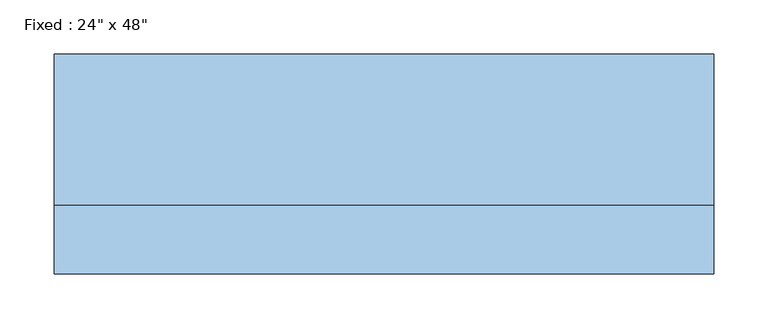
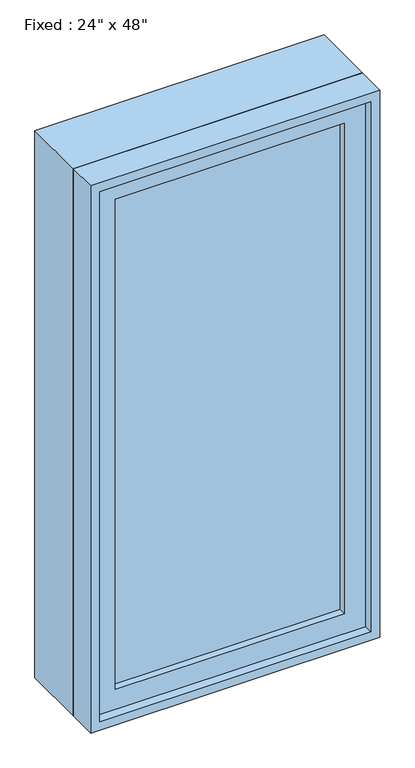
"""IFC4 building model written with IfcOpenShell, lengths in millimetres: window geometry."""

from ifc_helpers import new_model, si_unit, frame, origin, place, context, project, spatial, polyline, outline, extrude, source, transform, mapped, element, save


def window_9110666e(model_context):
    return source(origin(), model_context, "Body", "SweptSolid", [
        extrude(outline(polyline([(203.2, -53.975), (203.2, -66.675), (-279.4, -66.675), (-279.4, -53.975), (203.2, -53.975)])), frame((0.0, 0.0, 977.9), z_axis=(0.0, 0.0, 1.0), x_axis=(1.0, 0.0, 0.0)), (0.0, 0.0, 1.0), 1092.2),
        extrude(outline(polyline([(2114.55, -323.85), (933.45, -323.85), (933.45, 247.65), (2114.55, 247.65), (2114.55, -323.85)]), holes=[polyline([(2070.1, -279.4), (2070.1, 203.2), (977.9, 203.2), (977.9, -279.4), (2070.1, -279.4)])]), frame((0.0, -82.55, 0.0), z_axis=(0.0, 1.0, 0.0), x_axis=(0.0, 0.0, 1.0)), (0.0, 0.0, 1.0), 44.45),
        extrude(outline(polyline([(2133.6, -342.9), (914.4, -342.9), (914.4, 266.7), (2133.6, 266.7), (2133.6, -342.9)]), holes=[polyline([(2101.85, -311.15), (2101.85, 234.95), (946.15, 234.95), (946.15, -311.15), (2101.85, -311.15)])]), frame((0.0, -38.1, 0.0), z_axis=(0.0, 1.0, 0.0), x_axis=(0.0, 0.0, 1.0)), (0.0, 0.0, 1.0), 139.7),
        extrude(outline(polyline([(2133.6, 266.7), (2133.6, -342.9), (914.4, -342.9), (914.4, 266.7), (2133.6, 266.7)]), holes=[polyline([(2114.55, 247.65), (933.45, 247.65), (933.45, -323.85), (2114.55, -323.85), (2114.55, 247.65)])]), frame((0.0, -101.6, 0.0), z_axis=(0.0, 1.0, 0.0), x_axis=(0.0, 0.0, 1.0)), (0.0, 0.0, 1.0), 63.5),
    ])


if __name__ == "__main__":
    model = new_model("IFC4")
    model_context = context("Model", 3, world=origin())
    ifc_project = project(units=[si_unit("LENGTHUNIT", "METRE", prefix="MILLI")], contexts=[model_context])
    site = spatial("IfcSite", under=ifc_project)
    building = spatial("IfcBuilding", under=site)
    placement = place(None, origin())
    window_shape = window_9110666e(model_context)
    element("IfcWindow", 1, ObjectType="Fixed : 24\" x 48\"", at=placement, inside=building, context=model_context, shape_type="MappedRepresentation", body=[
        mapped(window_shape, transform((0.0, 0.0, 0.0), x_axis=(1.0, 0.0, 0.0), y_axis=(0.0, 1.0, 0.0), z_axis=(0.0, 0.0, 1.0))),
    ])
    save(model, "model.ifc")

# Revit data of these elements
# Type "Fixed : 24\" x 48\""
#   Type Mark = "2"
#   Construction Type Id = "GSP4R"
#   Assembly Code = "B2020100"
#   Analytic Construction = "1/8 in Pilkington single glazing"
#   Visual Light Transmittance = 0.9
#   Solar Heat Gain Coefficient = 0.78
#   Heat Transfer Coefficient (U) = 0.6496 BTU/(h·ft²·°F)
#   Height = 4' - 0"
#   Default Sill Height = 3' - 0"
#   Width = 2' - 0"
#   Window Inset = 0' - 0 3/4"
#   Define Thermal Properties by = 1
#   Glass Pane Material = Glass
#   Sash Material = Sash
#   Wall Closure = (empty or 0)
# Element 1 (IfcWindow, "Fixed : 24\" x 48\"")
#   Materials on its faces: "Sash", "Glass"
# Materials
#   "Glass": class "Glass", colour RGB 0 128 192, transparency 0.75, Description = "Soda Lime Glass", Cost = 0
#   "Sash": class "Wood", colour RGB 224 178 126, transparency 0
